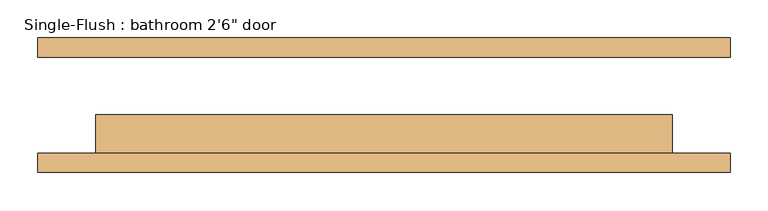
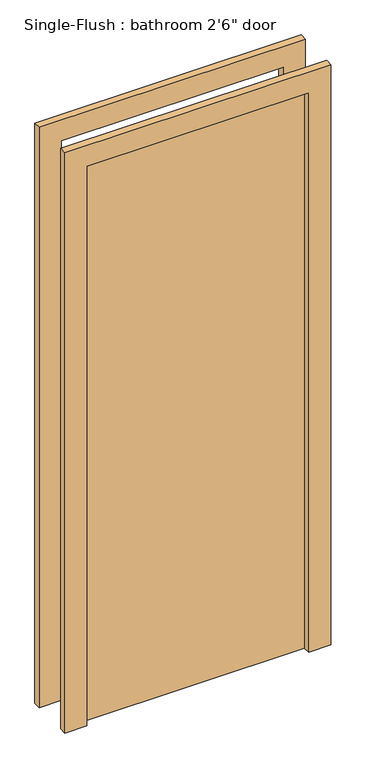
"""IFC4 building model written with IfcOpenShell, lengths in millimetres: door geometry."""

from ifc_helpers import new_model, si_unit, frame, origin, origin_with_axes, place, context, project, spatial, polyline, outline, extrude, source, transform, mapped, element, save


def door_e00f436c(model_context):
    return source(origin(), model_context, "Body", "SweptSolid", [
        extrude(outline(polyline([(2108.2, -457.2), (0.0, -457.2), (0.0, -381.0), (2032.0, -381.0), (2032.0, 381.0), (0.0, 381.0), (0.0, 457.2), (2108.2, 457.2), (2108.2, -457.2)])), frame((0.0, -88.9, 0.0), z_axis=(0.0, 1.0, 0.0), x_axis=(0.0, 0.0, 1.0)), (0.0, 0.0, 1.0), 25.4),
        extrude(outline(polyline([(2108.2, 457.2), (2108.2, -457.2), (0.0, -457.2), (0.0, -381.0), (2032.0, -381.0), (2032.0, 381.0), (0.0, 381.0), (0.0, 457.2), (2108.2, 457.2)])), frame((0.0, 63.5, 0.0), z_axis=(0.0, 1.0, 0.0), x_axis=(0.0, 0.0, 1.0)), (0.0, 0.0, 1.0), 25.4),
        extrude(outline(polyline([(381.0, -12.7), (381.0, -63.5), (-381.0, -63.5), (-381.0, -12.7), (381.0, -12.7)])), origin_with_axes(), (0.0, 0.0, 1.0), 2032.0),
    ])


if __name__ == "__main__":
    model = new_model("IFC4")
    model_context = context("Model", 3, world=origin())
    ifc_project = project(units=[si_unit("LENGTHUNIT", "METRE", prefix="MILLI")], contexts=[model_context])
    site = spatial("IfcSite", under=ifc_project)
    building = spatial("IfcBuilding", under=site)
    placement = place(None, origin())
    door_shape = door_e00f436c(model_context)
    element("IfcDoor", 1, ObjectType="Single-Flush : bathroom 2'6\" door", at=placement, inside=building, context=model_context, shape_type="MappedRepresentation", body=[
        mapped(door_shape, transform((0.0, 0.0, 0.0), x_axis=(1.0, 0.0, 0.0), y_axis=(0.0, 1.0, 0.0), z_axis=(0.0, 0.0, 1.0))),
    ])
    save(model, "model.ifc")

# Revit data of these elements
# Type "Single-Flush : bathroom 2'6\" door"
#   Type Mark = "12"
#   Construction Type Id = "MDOOR"
#   Assembly Code = "C1020"
#   Analytic Construction = "Metal"
#   Thickness = 0' - 2"
#   Heat Transfer Coefficient (U) = 0.651978 BTU/(h·ft²·°F)
#   Height = 6' - 8"
#   Trim Projection Ext = 0' - 1"
#   Trim Projection Int = 0' - 1"
#   Trim Width = 0' - 3"
#   Width = 2' - 6"
#   Define Thermal Properties by = 1
#   Door Material = Door - Panel
#   Frame Material = Door - Frame
#   Visual Light Transmittance = 0
#   Solar Heat Gain Coefficient = 0
#   Function = (empty or 0)
#   Wall Closure = (empty or 0)
# Element 1 (IfcDoor, "Single-Flush : bathroom 2'6\" door")
#   Materials on its faces: "Door - Frame", "Door - Panel"
# Materials
#   "Door - Panel": class "Wood", colour RGB 210 159 95, transparency 0, Cost = 0
#   "Door - Frame": colour RGB 118 70 51, transparency 0, Cost = 0
